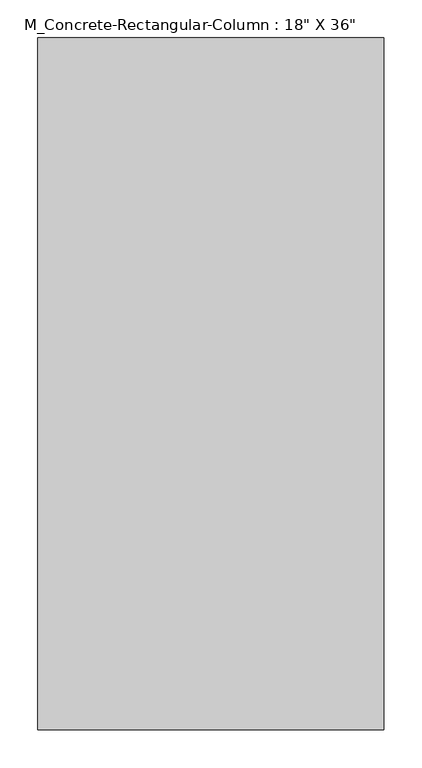
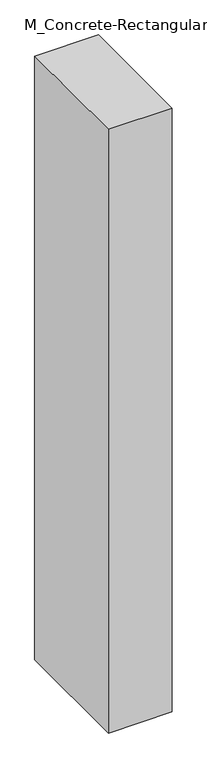
"""IFC4 building model written with IfcOpenShell, lengths in millimetres: column geometry."""

from ifc_helpers import new_model, si_unit, origin, origin_with_axes, place, context, project, spatial, polyline, outline, extrude, source, transform, mapped, element, save


def column_6107471e(model_context):
    return source(origin(), model_context, "Body", "SweptSolid", [
        extrude(outline(polyline([(228.6, 457.2), (228.6, -457.2), (-228.6, -457.2), (-228.6, 457.2), (228.6, 457.2)])), origin_with_axes(), (0.0, 0.0, 1.0), 4572.0),
    ])


if __name__ == "__main__":
    model = new_model("IFC4")
    model_context = context("Model", 3, world=origin())
    ifc_project = project(units=[si_unit("LENGTHUNIT", "METRE", prefix="MILLI")], contexts=[model_context])
    site = spatial("IfcSite", under=ifc_project)
    building = spatial("IfcBuilding", under=site)
    placement = place(None, origin())
    column_shape = column_6107471e(model_context)
    element("IfcColumn", 1, ObjectType="M_Concrete-Rectangular-Column : 18\" X 36\"", at=placement, inside=building, context=model_context, shape_type="MappedRepresentation", body=[
        mapped(column_shape, transform((0.0, 0.0, 0.0), x_axis=(1.0, 0.0, 0.0), y_axis=(0.0, 1.0, 0.0), z_axis=(0.0, 0.0, 1.0))),
    ])
    save(model, "model.ifc")

# Revit data of these elements
# Type "M_Concrete-Rectangular-Column : 18\" X 36\""
#   b = 457.2 mm
#   h = 914.4 mm
#   Structural Material [instance default] = Concrete, Cast-in-Place gray
# Element 1 (IfcColumn, "M_Concrete-Rectangular-Column : 18\" X 36\"")
#   Materials on its faces: "Concrete, Cast-in-Place gray"
# Materials
#   "Concrete, Cast-in-Place gray": class "Concrete", colour RGB 192 192 192, transparency 0, Description = "Cast-in-place concrete", Cost = 0
